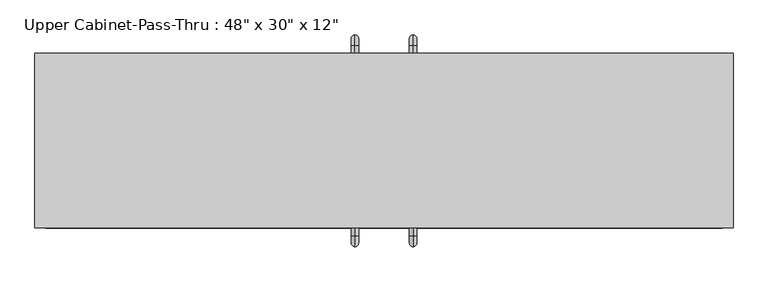
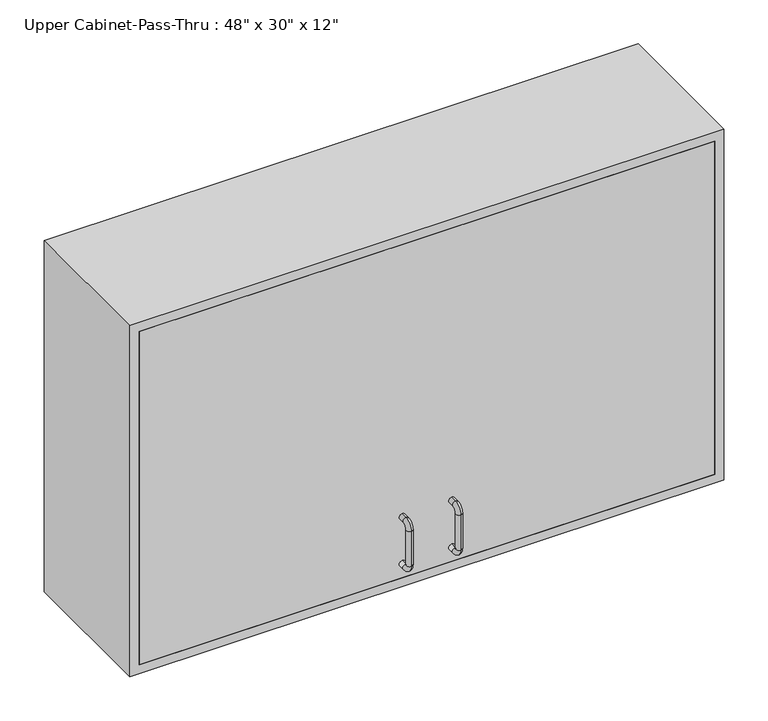
"""IFC4 building model written with IfcOpenShell, lengths in millimetres: furniture geometry."""

from ifc_helpers import new_model, si_unit, point, frame, origin, place, context, project, spatial, polyline, circle_curve, ellipse_curve, trimmed, outline, extrude, source, transform, mapped, element, save
from ifc_brep_helpers import plane_surface, cylinder_surface, revolved_surface, advanced_brep


def furniture_ea954fa4(model_context):
    return source(origin(), model_context, "Body", "SolidModel", [
        extrude(outline(polyline([(1371.6, 628.3377049), (2133.6, 628.3377049), (2133.6, -590.8622951), (1371.6, -590.8622951), (1371.6, 628.3377049)]), holes=[polyline([(1390.65, 609.2877049), (1390.65, -571.8122951), (2114.55, -571.8122951), (2114.55, 609.2877049), (1390.65, 609.2877049)])]), frame((0.0, -304.8, 0.0), z_axis=(0.0, 1.0, 0.0), x_axis=(0.0, 0.0, 1.0)), (0.0, 0.0, 1.0), 304.8),
        extrude(outline(polyline([(609.2877049, -19.05), (-571.8122951, -19.05), (-571.8122951, 0.0), (609.2877049, 0.0), (609.2877049, -19.05)])), frame((0.0, 0.0, 1390.65), z_axis=(0.0, 0.0, 1.0), x_axis=(1.0, 0.0, 0.0)), (0.0, 0.0, 1.0), 723.9),
        advanced_brep(
        [(69.5377049, -305.4314103, 1517.65), (69.5377049, -305.4314103, 1530.35), (69.5377049, -318.1314103, 1517.65), (69.5377049, -318.1314103, 1530.35), (69.5377049, -337.1814103, 1511.3), (69.5377049, -324.4814103, 1511.3), (69.5377049, -324.4814103, 1435.1), (69.5377049, -337.1814103, 1435.1), (69.5377049, -318.1314103, 1416.05), (69.5377049, -318.1314103, 1428.75), (69.5377049, -305.4314103, 1428.75), (69.5377049, -305.4314103, 1416.05)],
        [
            (0, 1, circle_curve(frame((69.5377049, -305.4314103, 1524.0), z_axis=(0.0, 1.0, 0.0), x_axis=(0.0, 0.0, 1.0)), 6.35)),
            (1, 0, circle_curve(frame((69.5377049, -305.4314103, 1524.0), z_axis=(0.0, 1.0, 0.0), x_axis=(0.0, 0.0, 1.0)), 6.35)),
            (0, 2),
            (2, 3, circle_curve(frame((69.5377049, -318.1314103, 1524.0), z_axis=(0.0, 1.0, 0.0), x_axis=(0.0, 0.0, 1.0)), 6.35)),
            (3, 1),
            (3, 2, circle_curve(frame((69.5377049, -318.1314103, 1524.0), z_axis=(0.0, 1.0, 0.0), x_axis=(0.0, 0.0, 1.0)), 6.35)),
            (4, 3, circle_curve(frame((69.5377049, -318.1314103, 1511.3), z_axis=(-1.0, 0.0, 0.0), x_axis=(0.0, 0.0, 1.0)), 19.05)),
            (2, 5, circle_curve(frame((69.5377049, -318.1314103, 1511.3), z_axis=(1.0, 0.0, 0.0), x_axis=(0.0, 0.0, 1.0)), 6.35)),
            (5, 4, circle_curve(frame((69.5377049, -330.8314103, 1511.3), z_axis=(0.0, 0.0, 1.0), x_axis=(0.0, -1.0, 0.0)), 6.35)),
            (4, 5, circle_curve(frame((69.5377049, -330.8314103, 1511.3), z_axis=(0.0, 0.0, 1.0), x_axis=(0.0, -1.0, 0.0)), 6.35)),
            (5, 6),
            (6, 7, circle_curve(frame((69.5377049, -330.8314103, 1435.1), z_axis=(0.0, 0.0, 1.0), x_axis=(0.0, -1.0, 0.0)), 6.35)),
            (7, 4),
            (7, 6, circle_curve(frame((69.5377049, -330.8314103, 1435.1), z_axis=(0.0, 0.0, 1.0), x_axis=(0.0, -1.0, 0.0)), 6.35)),
            (8, 7, circle_curve(frame((69.5377049, -318.1314103, 1435.1), z_axis=(-1.0, 0.0, 0.0), x_axis=(0.0, -1.0, 0.0)), 19.05)),
            (6, 9, circle_curve(frame((69.5377049, -318.1314103, 1435.1), z_axis=(1.0, 0.0, 0.0), x_axis=(0.0, -1.0, 0.0)), 6.35)),
            (9, 8, circle_curve(frame((69.5377049, -318.1314103, 1422.4), z_axis=(0.0, -1.0, 0.0), x_axis=(0.0, 0.0, -1.0)), 6.35)),
            (8, 9, circle_curve(frame((69.5377049, -318.1314103, 1422.4), z_axis=(0.0, -1.0, 0.0), x_axis=(0.0, 0.0, -1.0)), 6.35)),
            (10, 11, circle_curve(frame((69.5377049, -305.4314103, 1422.4), z_axis=(0.0, 1.0, 0.0), x_axis=(0.0, 0.0, -1.0)), 6.35)),
            (11, 10, circle_curve(frame((69.5377049, -305.4314103, 1422.4), z_axis=(0.0, 1.0, 0.0), x_axis=(0.0, 0.0, -1.0)), 6.35)),
            (9, 10),
            (11, 8),
        ],
        [
            plane_surface(frame((63.1877049, -305.4314103, 1524.0), z_axis=(0.0, 1.0, 0.0), x_axis=(0.0, 0.0, -1.0))),
            cylinder_surface(frame((69.5377049, -305.4314103, 1524.0), z_axis=(0.0, 1.0, 0.0), x_axis=(0.0, 0.0, 1.0)), 6.35),
            revolved_surface(trimmed(ellipse_curve(frame((69.5377049, -318.1314103, 1524.0), z_axis=(0.0, 1.0, 0.0), x_axis=(0.0, 0.0, 1.0)), 6.35, 6.35), [point((69.5377049, -318.1314103, 1517.65))], [point((69.5377049, -318.1314103, 1530.35))], True, "CARTESIAN"), (69.5377049, -318.1314103, 1511.3), (1.0, 0.0, 0.0)),
            revolved_surface(trimmed(ellipse_curve(frame((69.5377049, -318.1314103, 1524.0), z_axis=(0.0, 1.0, 0.0), x_axis=(0.0, 0.0, 1.0)), 6.35, 6.35), [point((69.5377049, -318.1314103, 1530.35))], [point((69.5377049, -318.1314103, 1517.65))], True, "CARTESIAN"), (69.5377049, -318.1314103, 1511.3), (1.0, 0.0, 0.0)),
            cylinder_surface(frame((69.5377049, -330.8314103, 1511.3), z_axis=(0.0, 0.0, 1.0), x_axis=(0.0, -1.0, 0.0)), 6.35),
            revolved_surface(trimmed(ellipse_curve(frame((69.5377049, -330.8314103, 1435.1), z_axis=(0.0, 0.0, 1.0), x_axis=(0.0, -1.0, 0.0)), 6.35, 6.35), [point((69.5377049, -324.4814103, 1435.1))], [point((69.5377049, -337.1814103, 1435.1))], True, "CARTESIAN"), (69.5377049, -318.1314103, 1435.1), (1.0, 0.0, 0.0)),
            revolved_surface(trimmed(ellipse_curve(frame((69.5377049, -330.8314103, 1435.1), z_axis=(0.0, 0.0, 1.0), x_axis=(0.0, -1.0, 0.0)), 6.35, 6.35), [point((69.5377049, -337.1814103, 1435.1))], [point((69.5377049, -324.4814103, 1435.1))], True, "CARTESIAN"), (69.5377049, -318.1314103, 1435.1), (1.0, 0.0, 0.0)),
            plane_surface(frame((63.1877049, -305.4314103, 1422.4), z_axis=(0.0, 1.0, 0.0), x_axis=(0.0, 0.0, 1.0))),
            cylinder_surface(frame((69.5377049, -318.1314103, 1422.4), z_axis=(0.0, -1.0, 0.0), x_axis=(0.0, 0.0, -1.0)), 6.35),
        ],
        [
            (0, [[1, 2]]),
            (1, [[-1, 3, 4, 5]]),
            (1, [[-2, -5, 6, -3]]),
            (2, [[7, -4, 8, 9]]),
            (3, [[-8, -6, -7, 10]]),
            (4, [[-9, 11, 12, 13]]),
            (4, [[-10, -13, 14, -11]]),
            (5, [[15, -12, 16, 17]]),
            (6, [[-16, -14, -15, 18]]),
            (7, [[19, 20]]),
            (8, [[-17, 21, -20, 22]]),
            (8, [[-18, -22, -19, -21]]),
        ],
    ),
        advanced_brep(
        [(-32.0622951, -305.4314103, 1517.65), (-32.0622951, -305.4314103, 1530.35), (-32.0622951, -318.1314103, 1517.65), (-32.0622951, -318.1314103, 1530.35), (-32.0622951, -337.1814103, 1511.3), (-32.0622951, -324.4814103, 1511.3), (-32.0622951, -324.4814103, 1435.1), (-32.0622951, -337.1814103, 1435.1), (-32.0622951, -318.1314103, 1416.05), (-32.0622951, -318.1314103, 1428.75), (-32.0622951, -305.4314103, 1428.75), (-32.0622951, -305.4314103, 1416.05)],
        [
            (0, 1, circle_curve(frame((-32.0622951, -305.4314103, 1524.0), z_axis=(0.0, 1.0, 0.0), x_axis=(0.0, 0.0, 1.0)), 6.35)),
            (1, 0, circle_curve(frame((-32.0622951, -305.4314103, 1524.0), z_axis=(0.0, 1.0, 0.0), x_axis=(0.0, 0.0, 1.0)), 6.35)),
            (0, 2),
            (2, 3, circle_curve(frame((-32.0622951, -318.1314103, 1524.0), z_axis=(0.0, 1.0, 0.0), x_axis=(0.0, 0.0, 1.0)), 6.35)),
            (3, 1),
            (3, 2, circle_curve(frame((-32.0622951, -318.1314103, 1524.0), z_axis=(0.0, 1.0, 0.0), x_axis=(0.0, 0.0, 1.0)), 6.35)),
            (4, 3, circle_curve(frame((-32.0622951, -318.1314103, 1511.3), z_axis=(-1.0, 0.0, 0.0), x_axis=(0.0, 0.0, 1.0)), 19.05)),
            (2, 5, circle_curve(frame((-32.0622951, -318.1314103, 1511.3), z_axis=(1.0, 0.0, 0.0), x_axis=(0.0, 0.0, 1.0)), 6.35)),
            (5, 4, circle_curve(frame((-32.0622951, -330.8314103, 1511.3), z_axis=(0.0, 0.0, 1.0), x_axis=(0.0, -1.0, 0.0)), 6.35)),
            (4, 5, circle_curve(frame((-32.0622951, -330.8314103, 1511.3), z_axis=(0.0, 0.0, 1.0), x_axis=(0.0, -1.0, 0.0)), 6.35)),
            (5, 6),
            (6, 7, circle_curve(frame((-32.0622951, -330.8314103, 1435.1), z_axis=(0.0, 0.0, 1.0), x_axis=(0.0, -1.0, 0.0)), 6.35)),
            (7, 4),
            (7, 6, circle_curve(frame((-32.0622951, -330.8314103, 1435.1), z_axis=(0.0, 0.0, 1.0), x_axis=(0.0, -1.0, 0.0)), 6.35)),
            (8, 7, circle_curve(frame((-32.0622951, -318.1314103, 1435.1), z_axis=(-1.0, 0.0, 0.0), x_axis=(0.0, -1.0, 0.0)), 19.05)),
            (6, 9, circle_curve(frame((-32.0622951, -318.1314103, 1435.1), z_axis=(1.0, 0.0, 0.0), x_axis=(0.0, -1.0, 0.0)), 6.35)),
            (9, 8, circle_curve(frame((-32.0622951, -318.1314103, 1422.4), z_axis=(0.0, -1.0, 0.0), x_axis=(0.0, 0.0, -1.0)), 6.35)),
            (8, 9, circle_curve(frame((-32.0622951, -318.1314103, 1422.4), z_axis=(0.0, -1.0, 0.0), x_axis=(0.0, 0.0, -1.0)), 6.35)),
            (10, 11, circle_curve(frame((-32.0622951, -305.4314103, 1422.4), z_axis=(0.0, 1.0, 0.0), x_axis=(0.0, 0.0, -1.0)), 6.35)),
            (11, 10, circle_curve(frame((-32.0622951, -305.4314103, 1422.4), z_axis=(0.0, 1.0, 0.0), x_axis=(0.0, 0.0, -1.0)), 6.35)),
            (9, 10),
            (11, 8),
        ],
        [
            plane_surface(frame((-37.6086081, -305.4314103, 1524.0), z_axis=(0.0, 1.0, 0.0), x_axis=(0.0, 0.0, -1.0))),
            cylinder_surface(frame((-32.0622951, -305.4314103, 1524.0), z_axis=(0.0, 1.0, 0.0), x_axis=(0.0, 0.0, 1.0)), 6.35),
            revolved_surface(trimmed(ellipse_curve(frame((-32.0622951, -318.1314103, 1524.0), z_axis=(0.0, 1.0, 0.0), x_axis=(0.0, 0.0, 1.0)), 6.35, 6.35), [point((-32.0622951, -318.1314103, 1517.65))], [point((-32.0622951, -318.1314103, 1530.35))], True, "CARTESIAN"), (69.5377049, -318.1314103, 1511.3), (1.0, 0.0, 0.0)),
            revolved_surface(trimmed(ellipse_curve(frame((-32.0622951, -318.1314103, 1524.0), z_axis=(0.0, 1.0, 0.0), x_axis=(0.0, 0.0, 1.0)), 6.35, 6.35), [point((-32.0622951, -318.1314103, 1530.35))], [point((-32.0622951, -318.1314103, 1517.65))], True, "CARTESIAN"), (69.5377049, -318.1314103, 1511.3), (1.0, 0.0, 0.0)),
            cylinder_surface(frame((-32.0622951, -330.8314103, 1511.3), z_axis=(0.0, 0.0, 1.0), x_axis=(0.0, -1.0, 0.0)), 6.35),
            revolved_surface(trimmed(ellipse_curve(frame((-32.0622951, -330.8314103, 1435.1), z_axis=(0.0, 0.0, 1.0), x_axis=(0.0, -1.0, 0.0)), 6.35, 6.35), [point((-32.0622951, -324.4814103, 1435.1))], [point((-32.0622951, -337.1814103, 1435.1))], True, "CARTESIAN"), (69.5377049, -318.1314103, 1435.1), (1.0, 0.0, 0.0)),
            revolved_surface(trimmed(ellipse_curve(frame((-32.0622951, -330.8314103, 1435.1), z_axis=(0.0, 0.0, 1.0), x_axis=(0.0, -1.0, 0.0)), 6.35, 6.35), [point((-32.0622951, -337.1814103, 1435.1))], [point((-32.0622951, -324.4814103, 1435.1))], True, "CARTESIAN"), (69.5377049, -318.1314103, 1435.1), (1.0, 0.0, 0.0)),
            plane_surface(frame((-37.6086081, -305.4314103, 1422.4), z_axis=(0.0, 1.0, 0.0), x_axis=(0.0, 0.0, 1.0))),
            cylinder_surface(frame((-32.0622951, -318.1314103, 1422.4), z_axis=(0.0, -1.0, 0.0), x_axis=(0.0, 0.0, -1.0)), 6.35),
        ],
        [
            (0, [[1, 2]]),
            (1, [[-1, 3, 4, 5]]),
            (1, [[-2, -5, 6, -3]]),
            (2, [[7, -4, 8, 9]]),
            (3, [[-8, -6, -7, 10]]),
            (4, [[-9, 11, 12, 13]]),
            (4, [[-10, -13, 14, -11]]),
            (5, [[15, -12, 16, 17]]),
            (6, [[-16, -14, -15, 18]]),
            (7, [[19, 20]]),
            (8, [[-17, 21, -20, 22]]),
            (8, [[-18, -22, -19, -21]]),
        ],
    ),
        advanced_brep(
        [(69.5377049, 0.6314103, 1517.65), (69.5377049, 0.6314103, 1530.35), (69.5377049, 13.3314103, 1517.65), (69.5377049, 13.3314103, 1530.35), (69.5377049, 32.3814103, 1511.3), (69.5377049, 19.6814103, 1511.3), (69.5377049, 19.6814103, 1435.1), (69.5377049, 32.3814103, 1435.1), (69.5377049, 13.3314103, 1416.05), (69.5377049, 13.3314103, 1428.75), (69.5377049, 0.6314103, 1428.75), (69.5377049, 0.6314103, 1416.05)],
        [
            (0, 1, circle_curve(frame((69.5377049, 0.6314103, 1524.0), z_axis=(0.0, -1.0, 0.0), x_axis=(0.0, 0.0, -1.0)), 6.35)),
            (1, 0, circle_curve(frame((69.5377049, 0.6314103, 1524.0), z_axis=(0.0, -1.0, 0.0), x_axis=(0.0, 0.0, -1.0)), 6.35)),
            (0, 2),
            (2, 3, circle_curve(frame((69.5377049, 13.3314103, 1524.0), z_axis=(0.0, -1.0, 0.0), x_axis=(0.0, 0.0, -1.0)), 6.35)),
            (3, 1),
            (3, 2, circle_curve(frame((69.5377049, 13.3314103, 1524.0), z_axis=(0.0, -1.0, 0.0), x_axis=(0.0, 0.0, -1.0)), 6.35)),
            (4, 3, circle_curve(frame((69.5377049, 13.3314103, 1511.3), z_axis=(1.0, 0.0, 0.0), x_axis=(0.0, 0.0, 1.0)), 19.05)),
            (2, 5, circle_curve(frame((69.5377049, 13.3314103, 1511.3), z_axis=(-1.0, 0.0, 0.0), x_axis=(0.0, 0.0, 1.0)), 6.35)),
            (5, 4, circle_curve(frame((69.5377049, 26.0314103, 1511.3), z_axis=(0.0, 0.0, 1.0), x_axis=(0.0, -1.0, 0.0)), 6.35)),
            (4, 5, circle_curve(frame((69.5377049, 26.0314103, 1511.3), z_axis=(0.0, 0.0, 1.0), x_axis=(0.0, -1.0, 0.0)), 6.35)),
            (5, 6),
            (6, 7, circle_curve(frame((69.5377049, 26.0314103, 1435.1), z_axis=(0.0, 0.0, 1.0), x_axis=(0.0, -1.0, 0.0)), 6.35)),
            (7, 4),
            (7, 6, circle_curve(frame((69.5377049, 26.0314103, 1435.1), z_axis=(0.0, 0.0, 1.0), x_axis=(0.0, -1.0, 0.0)), 6.35)),
            (8, 7, circle_curve(frame((69.5377049, 13.3314103, 1435.1), z_axis=(1.0, 0.0, 0.0), x_axis=(0.0, 1.0, 0.0)), 19.05)),
            (6, 9, circle_curve(frame((69.5377049, 13.3314103, 1435.1), z_axis=(-1.0, 0.0, 0.0), x_axis=(0.0, 1.0, 0.0)), 6.35)),
            (9, 8, circle_curve(frame((69.5377049, 13.3314103, 1422.4), z_axis=(0.0, 1.0, 0.0), x_axis=(0.0, 0.0, 1.0)), 6.35)),
            (8, 9, circle_curve(frame((69.5377049, 13.3314103, 1422.4), z_axis=(0.0, 1.0, 0.0), x_axis=(0.0, 0.0, 1.0)), 6.35)),
            (10, 11, circle_curve(frame((69.5377049, 0.6314103, 1422.4), z_axis=(0.0, -1.0, 0.0), x_axis=(0.0, 0.0, 1.0)), 6.35)),
            (11, 10, circle_curve(frame((69.5377049, 0.6314103, 1422.4), z_axis=(0.0, -1.0, 0.0), x_axis=(0.0, 0.0, 1.0)), 6.35)),
            (9, 10),
            (11, 8),
        ],
        [
            plane_surface(frame((63.1877049, 0.6314103, 1524.0), z_axis=(0.0, -1.0, 0.0), x_axis=(0.0, 0.0, 1.0))),
            cylinder_surface(frame((69.5377049, 0.6314103, 1524.0), z_axis=(0.0, -1.0, 0.0), x_axis=(0.0, 0.0, -1.0)), 6.35),
            revolved_surface(trimmed(ellipse_curve(frame((69.5377049, 13.3314103, 1524.0), z_axis=(0.0, -1.0, 0.0), x_axis=(0.0, 0.0, -1.0)), 6.35, 6.35), [point((69.5377049, 13.3314103, 1517.65))], [point((69.5377049, 13.3314103, 1530.35))], True, "CARTESIAN"), (69.5377049, 13.3314103, 1511.3), (-1.0, 0.0, 0.0)),
            revolved_surface(trimmed(ellipse_curve(frame((69.5377049, 13.3314103, 1524.0), z_axis=(0.0, -1.0, 0.0), x_axis=(0.0, 0.0, -1.0)), 6.35, 6.35), [point((69.5377049, 13.3314103, 1530.35))], [point((69.5377049, 13.3314103, 1517.65))], True, "CARTESIAN"), (69.5377049, 13.3314103, 1511.3), (-1.0, 0.0, 0.0)),
            cylinder_surface(frame((69.5377049, 26.0314103, 1511.3), z_axis=(0.0, 0.0, 1.0), x_axis=(0.0, -1.0, 0.0)), 6.35),
            revolved_surface(trimmed(ellipse_curve(frame((69.5377049, 26.0314103, 1435.1), z_axis=(0.0, 0.0, 1.0), x_axis=(0.0, -1.0, 0.0)), 6.35, 6.35), [point((69.5377049, 19.6814103, 1435.1))], [point((69.5377049, 32.3814103, 1435.1))], True, "CARTESIAN"), (69.5377049, 13.3314103, 1435.1), (-1.0, 0.0, 0.0)),
            revolved_surface(trimmed(ellipse_curve(frame((69.5377049, 26.0314103, 1435.1), z_axis=(0.0, 0.0, 1.0), x_axis=(0.0, -1.0, 0.0)), 6.35, 6.35), [point((69.5377049, 32.3814103, 1435.1))], [point((69.5377049, 19.6814103, 1435.1))], True, "CARTESIAN"), (69.5377049, 13.3314103, 1435.1), (-1.0, 0.0, 0.0)),
            plane_surface(frame((63.1877049, 0.6314103, 1422.4), z_axis=(0.0, -1.0, 0.0), x_axis=(0.0, 0.0, -1.0))),
            cylinder_surface(frame((69.5377049, 13.3314103, 1422.4), z_axis=(0.0, 1.0, 0.0), x_axis=(0.0, 0.0, 1.0)), 6.35),
        ],
        [
            (0, [[1, 2]]),
            (1, [[-1, 3, 4, 5]]),
            (1, [[-2, -5, 6, -3]]),
            (2, [[7, -4, 8, 9]]),
            (3, [[-8, -6, -7, 10]]),
            (4, [[-9, 11, 12, 13]]),
            (4, [[-10, -13, 14, -11]]),
            (5, [[15, -12, 16, 17]]),
            (6, [[-16, -14, -15, 18]]),
            (7, [[19, 20]]),
            (8, [[-17, 21, -20, 22]]),
            (8, [[-18, -22, -19, -21]]),
        ],
    ),
        advanced_brep(
        [(-32.0622951, 0.6314103, 1518.3611126), (-32.0622951, 0.6314103, 1531.0611126), (-32.0622951, 13.3314103, 1518.3611126), (-32.0622951, 13.3314103, 1531.0611126), (-32.0622951, 32.3814103, 1512.0111126), (-32.0622951, 19.6814103, 1512.0111126), (-32.0622951, 19.6814103, 1435.8111126), (-32.0622951, 32.3814103, 1435.8111126), (-32.0622951, 13.3314103, 1416.7611126), (-32.0622951, 13.3314103, 1429.4611126), (-32.0622951, 0.6314103, 1429.4611126), (-32.0622951, 0.6314103, 1416.7611126)],
        [
            (0, 1, circle_curve(frame((-32.0622951, 0.6314103, 1524.7111126), z_axis=(0.0, -1.0, 0.0), x_axis=(0.0, 0.0, -1.0)), 6.35)),
            (1, 0, circle_curve(frame((-32.0622951, 0.6314103, 1524.7111126), z_axis=(0.0, -1.0, 0.0), x_axis=(0.0, 0.0, -1.0)), 6.35)),
            (0, 2),
            (2, 3, circle_curve(frame((-32.0622951, 13.3314103, 1524.7111126), z_axis=(0.0, -1.0, 0.0), x_axis=(0.0, 0.0, -1.0)), 6.35)),
            (3, 1),
            (3, 2, circle_curve(frame((-32.0622951, 13.3314103, 1524.7111126), z_axis=(0.0, -1.0, 0.0), x_axis=(0.0, 0.0, -1.0)), 6.35)),
            (4, 3, circle_curve(frame((-32.0622951, 13.3314103, 1512.0111126), z_axis=(1.0, 0.0, 0.0), x_axis=(0.0, 0.0, 1.0)), 19.05)),
            (2, 5, circle_curve(frame((-32.0622951, 13.3314103, 1512.0111126), z_axis=(-1.0, 0.0, 0.0), x_axis=(0.0, 0.0, 1.0)), 6.35)),
            (5, 4, circle_curve(frame((-32.0622951, 26.0314103, 1512.0111126), z_axis=(0.0, 0.0, 1.0), x_axis=(0.0, -1.0, 0.0)), 6.35)),
            (4, 5, circle_curve(frame((-32.0622951, 26.0314103, 1512.0111126), z_axis=(0.0, 0.0, 1.0), x_axis=(0.0, -1.0, 0.0)), 6.35)),
            (5, 6),
            (6, 7, circle_curve(frame((-32.0622951, 26.0314103, 1435.8111126), z_axis=(0.0, 0.0, 1.0), x_axis=(0.0, -1.0, 0.0)), 6.35)),
            (7, 4),
            (7, 6, circle_curve(frame((-32.0622951, 26.0314103, 1435.8111126), z_axis=(0.0, 0.0, 1.0), x_axis=(0.0, -1.0, 0.0)), 6.35)),
            (8, 7, circle_curve(frame((-32.0622951, 13.3314103, 1435.8111126), z_axis=(1.0, 0.0, 0.0), x_axis=(0.0, 1.0, 0.0)), 19.05)),
            (6, 9, circle_curve(frame((-32.0622951, 13.3314103, 1435.8111126), z_axis=(-1.0, 0.0, 0.0), x_axis=(0.0, 1.0, 0.0)), 6.35)),
            (9, 8, circle_curve(frame((-32.0622951, 13.3314103, 1423.1111126), z_axis=(0.0, 1.0, 0.0), x_axis=(0.0, 0.0, 1.0)), 6.35)),
            (8, 9, circle_curve(frame((-32.0622951, 13.3314103, 1423.1111126), z_axis=(0.0, 1.0, 0.0), x_axis=(0.0, 0.0, 1.0)), 6.35)),
            (10, 11, circle_curve(frame((-32.0622951, 0.6314103, 1423.1111126), z_axis=(0.0, -1.0, 0.0), x_axis=(0.0, 0.0, 1.0)), 6.35)),
            (11, 10, circle_curve(frame((-32.0622951, 0.6314103, 1423.1111126), z_axis=(0.0, -1.0, 0.0), x_axis=(0.0, 0.0, 1.0)), 6.35)),
            (9, 10),
            (11, 8),
        ],
        [
            plane_surface(frame((-37.6086081, 0.6314103, 1524.7111126), z_axis=(0.0, -1.0, 0.0), x_axis=(0.0, 0.0, 1.0))),
            cylinder_surface(frame((-32.0622951, 0.6314103, 1524.7111126), z_axis=(0.0, -1.0, 0.0), x_axis=(0.0, 0.0, -1.0)), 6.35),
            revolved_surface(trimmed(ellipse_curve(frame((-32.0622951, 13.3314103, 1524.7111126), z_axis=(0.0, -1.0, 0.0), x_axis=(0.0, 0.0, -1.0)), 6.35, 6.35), [point((-32.0622951, 13.3314103, 1518.3611126))], [point((-32.0622951, 13.3314103, 1531.0611126))], True, "CARTESIAN"), (69.5377049, 13.3314103, 1512.0111126), (-1.0, 0.0, 0.0)),
            revolved_surface(trimmed(ellipse_curve(frame((-32.0622951, 13.3314103, 1524.7111126), z_axis=(0.0, -1.0, 0.0), x_axis=(0.0, 0.0, -1.0)), 6.35, 6.35), [point((-32.0622951, 13.3314103, 1531.0611126))], [point((-32.0622951, 13.3314103, 1518.3611126))], True, "CARTESIAN"), (69.5377049, 13.3314103, 1512.0111126), (-1.0, 0.0, 0.0)),
            cylinder_surface(frame((-32.0622951, 26.0314103, 1512.0111126), z_axis=(0.0, 0.0, 1.0), x_axis=(0.0, -1.0, 0.0)), 6.35),
            revolved_surface(trimmed(ellipse_curve(frame((-32.0622951, 26.0314103, 1435.8111126), z_axis=(0.0, 0.0, 1.0), x_axis=(0.0, -1.0, 0.0)), 6.35, 6.35), [point((-32.0622951, 19.6814103, 1435.8111126))], [point((-32.0622951, 32.3814103, 1435.8111126))], True, "CARTESIAN"), (69.5377049, 13.3314103, 1435.8111126), (-1.0, 0.0, 0.0)),
            revolved_surface(trimmed(ellipse_curve(frame((-32.0622951, 26.0314103, 1435.8111126), z_axis=(0.0, 0.0, 1.0), x_axis=(0.0, -1.0, 0.0)), 6.35, 6.35), [point((-32.0622951, 32.3814103, 1435.8111126))], [point((-32.0622951, 19.6814103, 1435.8111126))], True, "CARTESIAN"), (69.5377049, 13.3314103, 1435.8111126), (-1.0, 0.0, 0.0)),
            plane_surface(frame((-37.6086081, 0.6314103, 1423.1111126), z_axis=(0.0, -1.0, 0.0), x_axis=(0.0, 0.0, -1.0))),
            cylinder_surface(frame((-32.0622951, 13.3314103, 1423.1111126), z_axis=(0.0, 1.0, 0.0), x_axis=(0.0, 0.0, 1.0)), 6.35),
        ],
        [
            (0, [[1, 2]]),
            (1, [[-1, 3, 4, 5]]),
            (1, [[-2, -5, 6, -3]]),
            (2, [[7, -4, 8, 9]]),
            (3, [[-8, -6, -7, 10]]),
            (4, [[-9, 11, 12, 13]]),
            (4, [[-10, -13, 14, -11]]),
            (5, [[15, -12, 16, 17]]),
            (6, [[-16, -14, -15, 18]]),
            (7, [[19, 20]]),
            (8, [[-17, 21, -20, 22]]),
            (8, [[-18, -22, -19, -21]]),
        ],
    ),
        extrude(outline(polyline([(609.2877049, -304.8), (-571.8122951, -304.8), (-571.8122951, -285.75), (609.2877049, -285.75), (609.2877049, -304.8)])), frame((0.0, 0.0, 1390.65), z_axis=(0.0, 0.0, 1.0), x_axis=(1.0, 0.0, 0.0)), (0.0, 0.0, 1.0), 723.9),
    ])


if __name__ == "__main__":
    model = new_model("IFC4")
    model_context = context("Model", 3, world=origin())
    ifc_project = project(units=[si_unit("LENGTHUNIT", "METRE", prefix="MILLI")], contexts=[model_context])
    site = spatial("IfcSite", under=ifc_project)
    building = spatial("IfcBuilding", under=site)
    placement = place(None, origin())
    furniture_shape = furniture_ea954fa4(model_context)
    element("IfcFurniture", 1, ObjectType="Upper Cabinet-Pass-Thru : 48\" x 30\" x 12\"", at=placement, inside=building, context=model_context, shape_type="MappedRepresentation", body=[
        mapped(furniture_shape, transform((0.0, 0.0, 0.0), x_axis=(1.0, 0.0, 0.0), y_axis=(0.0, 1.0, 0.0), z_axis=(0.0, 0.0, 1.0))),
    ])
    save(model, "model.ifc")

# Revit data of these elements
# Type "Upper Cabinet-Pass-Thru : 48\" x 30\" x 12\""
#   Depth = 1' - 0"
#   Height = 2' - 6"
#   Top of Cabinet = 7' - 0"
#   Width = 4' - 0"
#   Default Elevation = 0
# Element 1 (IfcFurniture, "Upper Cabinet-Pass-Thru : 48\" x 30\" x 12\"")
#   Materials on its faces: "Cabinet"
# Materials
#   "Cabinet": colour RGB 204 122 2, transparency 0
